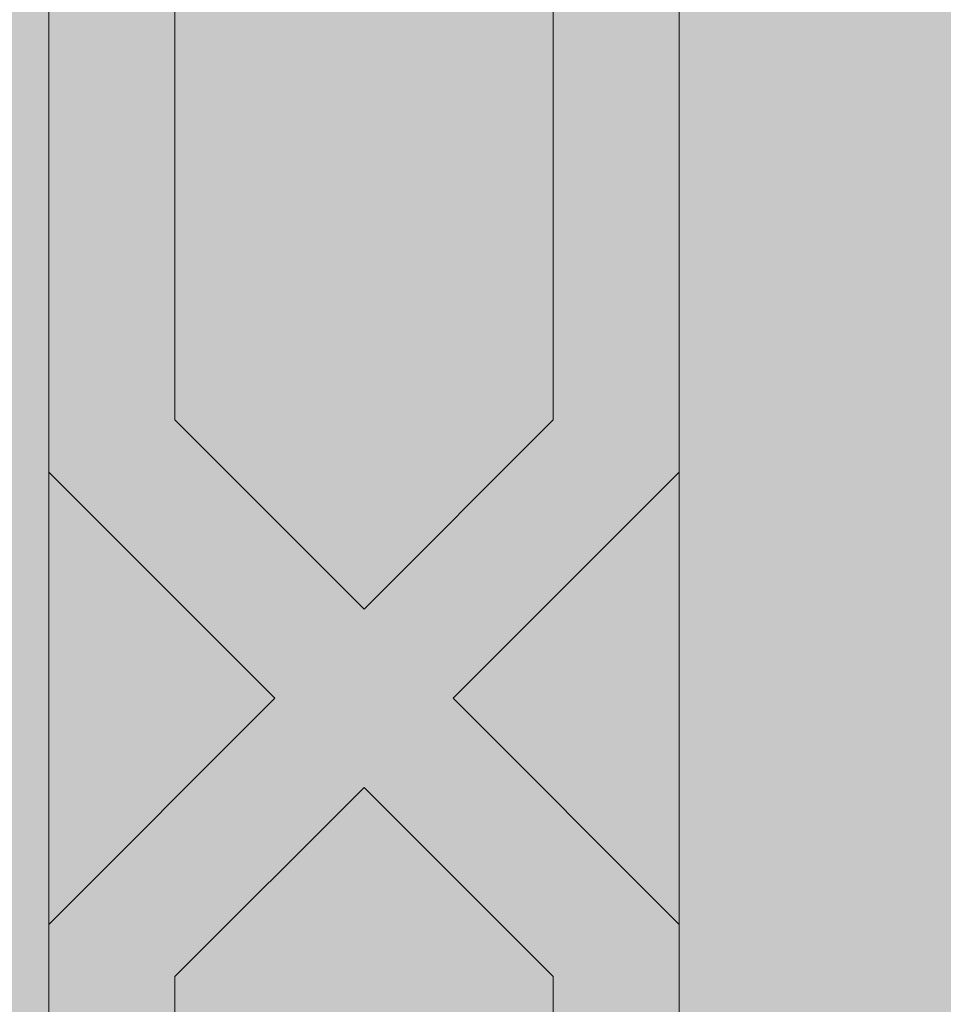
# Model space of a CAD drawing. Units: inches. Extents: x 844 to 2234, y 346 to 1084.
# Tile 17 of 93: x 1116.421 to 1118.29, y 701.25 to 703.242. Entities that reach past the tile are written whole.
import ezdxf

# ---------------------------------------------------------------- set-up
doc = ezdxf.new("R2010")
doc.units = ezdxf.units.IN
doc.header["$MEASUREMENT"] = 0
for name, color, linetype, lineweight in [('A-ANNO-DIMS', 2, 'Continuous', 18), ('furniture', 8, 'Continuous', 18), ('RA-AP-01$0$INT', 35, 'Continuous', 5)]:
    doc.layers.add(name, color=color, linetype=linetype, lineweight=lineweight)
doc.layers.add('RA-AP-01$0$FURN', color=3, linetype='Continuous')
doc.styles.get("Standard").update_dxf_attribs({"font": 'arial.ttf'})
doc.dimstyles.get("Standard").update_dxf_attribs({"dimtxt": 6, "dimasz": 3, "dimexe": 0.18, "dimexo": 0.0625, "dimgap": 0.09, "dimtad": 0, "dimtih": 1, "dimtoh": 1, "dimdec": 1, "dimzin": 0, "dimdsep": 46, "dimlunit": 3, "dimtxsty": 'Standard', "dimblk": 'ARCHTICK', "dimcen": 0.09, "dimadec": 0, "dimazin": 0, "dimtfac": 1, "dimtdec": 1, "dimtofl": 0, "dimtmove": 0, "dimatfit": 3, "dimfxl": 1, "dimtolj": 1, "dimtzin": 0, "dimarcsym": 0})

# ---------------------------------------------------------------- blocks, each defined once
blk = doc.blocks.new('A$C18D01794')
at = {"layer": 'RA-AP-01$0$INT'}
h = blk.add_hatch(color=256, dxfattribs=at)
h.paths.add_polyline_path([(4.355206456958071, -6.156712009588037), (4.355206456958071, -8.056712009588038), (5.455206456958072, -8.056712009588038), (5.455206456958072, -6.156712009588037)])
h.paths.add_polyline_path([(4.405206456958072, -8.006712009588039), (4.405206456958072, -6.206712009588038), (5.405206456958072, -6.206712009588038), (5.405206456958072, -8.006712009588039)], flags=16)
h = blk.add_hatch(color=256, dxfattribs=at)
h.paths.add_polyline_path([(4.505206456958071, -7.585498806127123), (4.46934859260189, -7.549640941759413), (4.505206456958071, -7.513783077414768), (4.505206456958071, -7.381963272220687), (4.469348592616735, -7.346105407867824), (4.505206456958071, -7.310247543514964), (4.505206456958071, -7.178427738324996), (4.469348592586679, -7.142569873965138), (4.505206456952245, -7.106712009588038), (4.476922185709333, -7.106712009588038), (4.455206456960671, -7.128427738343681), (4.433490728198047, -7.106712009588038), (4.405206456946033, -7.106712009588036), (4.441064321339216, -7.142569873969684), (4.40520645695807, -7.178427738362358), (4.405206456958072, -7.310247543472698), (4.441064321364728, -7.346105407867826), (4.40520645695807, -7.381963272262947), (4.40520645695807, -7.513783077378263), (4.441064321354429, -7.549640941786153), (4.405206456958072, -7.585498806170974), (4.405206456958072, -7.717318611286652), (4.441064321333084, -7.753176475673194), (4.405206456958072, -7.789034340036673), (4.405206456958072, -8.006712009588039), (4.644348592588106, -8.006712009588039), (4.680206456964639, -7.970854145211967), (4.716064321341165, -8.006712009588039), (4.869348592586113, -8.006712009588039), (4.905206456964143, -7.970854145210465), (4.941064321342174, -8.006712009588039), (5.094348592587118, -8.006712009588037), (5.130206456963649, -7.970854145211967), (5.166064321340178, -8.006712009588039), (5.405206456958072, -8.006712009588039), (5.405206456958072, -7.789034340024526), (5.369348592595202, -7.753176475673196), (5.40520645695807, -7.717318611298797), (5.40520645695807, -7.585498806158829), (5.369348592573859, -7.549640941786151), (5.40520645695807, -7.51378307739041), (5.40520645695807, -7.381963272250803), (5.36934859256356, -7.346105407867824), (5.405206456958072, -7.310247543484846), (5.405206456958072, -7.178427738350217), (5.369348592589068, -7.142569873969682), (5.405206456982249, -7.106712009588038), (5.376922185730244, -7.106712009588038), (5.355206456967613, -7.128427738343679), (5.333490728218955, -7.10671200958804), (5.305206456976043, -7.106712009588042), (5.341064321341609, -7.142569873965136), (5.305206456958072, -7.178427738337141), (5.305206456958072, -7.310247543502816), (5.34106432131155, -7.346105407867824), (5.305206456958072, -7.381963272232832), (5.30520645695807, -7.513783077402624), (5.341064321326395, -7.549640941759413), (5.305206456958072, -7.585498806139263), (5.305206456958072, -7.717318611299605), (5.341064321347738, -7.753176475677737), (5.305206456958072, -7.78903434007894), (5.30520645695807, -7.906712009588039), (5.166064321336834, -7.906712009588039), (5.130206456963647, -7.942569873961684), (5.094348592590464, -7.906712009588039), (4.941064321338827, -7.906712009588041), (4.905206456964145, -7.942569873963183), (4.869348592589459, -7.906712009588039), (4.716064321337822, -7.906712009588041), (4.680206456964641, -7.942569873961684), (4.644348592591453, -7.906712009588039), (4.505206456958071, -7.906712009588039), (4.505206456958071, -7.789034340066795), (4.469348592580545, -7.753176475677738), (4.505206456958071, -7.717318611311748)])
h.paths.add_polyline_path([(4.485206456974132, -7.709034340046354), (4.45520645695909, -7.739034340051736), (4.425206456974128, -7.709034340057131), (4.425206456993394, -7.593783077384998), (4.45520645699153, -7.563783077396511), (4.485206456993396, -7.593783077408017)], flags=16)
h.paths.add_polyline_path([(4.455206456954537, -7.767318611299197), (4.485206456958242, -7.797318611312542), (4.48520645695951, -7.912569873958716), (4.45520645695415, -7.942569873954422), (4.425206456957888, -7.912569873967813), (4.425206456957888, -7.797318611286197)], flags=16)
h.paths.add_polyline_path([(4.455206456964794, -7.535498806149051), (4.42520645696469, -7.5054988061393), (4.425206456983954, -7.390247543486406), (4.455206456990734, -7.360247543489279), (4.485206456983953, -7.39024754349214), (4.485206456964687, -7.505498806158811)], flags=16)
h.paths.add_polyline_path([(4.499348592588947, -7.926712009585049), (4.636064321340932, -7.926712009585049), (4.666064321342317, -7.956712009586821), (4.636064321343707, -7.986712009585048), (4.499348592575121, -7.986712009585048), (4.469348592591685, -7.956712009591957)], flags=16)
h.paths.add_polyline_path([(4.425206456957888, -7.940854145195974), (4.471064321332215, -7.986712009585049), (4.425206456957888, -7.986712009585049)], flags=16)
h.paths.add_polyline_path([(4.455206456990734, -7.331963272246367), (4.425206456989053, -7.301963272254337), (4.425206456969784, -7.186712009596224), (4.455206456965226, -7.156712009591144), (4.485206456969787, -7.186712009586051), (4.485206456989053, -7.301963272238404)], flags=16)
h.paths.add_polyline_path([(4.72434859258714, -7.926712009586255), (4.861064321340141, -7.926712009586248), (4.891064321340324, -7.956712009586823), (4.861064321340513, -7.986712009586252), (4.724348592586768, -7.986712009586252), (4.694348592586956, -7.956712009586821)], flags=16)
h.paths.add_polyline_path([(4.919348592587961, -7.956712009586821), (4.949348592588145, -7.92671200958625), (5.08606432134115, -7.926712009586253), (5.116064321341327, -7.956712009586823), (5.086064321341519, -7.986712009586252), (4.949348592587774, -7.986712009586252)], flags=16)
h.paths.add_polyline_path([(5.144348592585967, -7.956712009586823), (5.174348592587358, -7.926712009585049), (5.311064321339338, -7.926712009585049), (5.3410643213366, -7.956712009591957), (5.311064321353163, -7.986712009585048), (5.174348592584576, -7.986712009585048)], flags=16)
h.paths.add_polyline_path([(5.32520645693489, -7.593783077408021), (5.355206456936755, -7.563783077396511), (5.385206456934894, -7.593783077384998), (5.38520645695416, -7.709034340057128), (5.355206456969194, -7.739034340051736), (5.325206456954153, -7.709034340046352)], flags=16)
h.paths.add_polyline_path([(5.325206456970042, -7.797318611312542), (5.355206456973747, -7.767318611299197), (5.385206456970398, -7.7973186112862), (5.385206456970398, -7.912569873967816), (5.355206456974136, -7.942569873954422), (5.325206456968778, -7.912569873958716)], flags=16)
h.paths.add_polyline_path([(5.325206456963599, -7.505498806158811), (5.325206456944333, -7.39024754349214), (5.355206456937552, -7.360247543489279), (5.385206456944332, -7.39024754348641), (5.385206456963596, -7.505498806139303), (5.355206456963492, -7.53549880614905)], flags=16)
h.paths.add_polyline_path([(5.32520645693923, -7.301963272238403), (5.3252064569585, -7.186712009586051), (5.355206456963062, -7.156712009591142), (5.3852064569585, -7.186712009596224), (5.385206456939234, -7.301963272254338), (5.355206456937552, -7.331963272246369)], flags=16)
h.paths.add_polyline_path([(5.339348592596071, -7.986712009585048), (5.385206456970398, -7.940854145195972), (5.385206456970396, -7.986712009585048)], flags=16)
h = blk.add_hatch(color=256, dxfattribs=at)
h.paths.add_polyline_path([(4.469348592586677, -7.142569873965136), (4.505206456958073, -7.178427738324996), (4.505206456958071, -7.106712009582215)])
h.paths.add_polyline_path([(4.455206456960671, -7.128427738343681), (4.476922185709333, -7.106712009588038), (4.433490728198045, -7.106712009588038)])
h.paths.add_polyline_path([(4.405206456958073, -7.178427738362358), (4.441064321339218, -7.142569873969684), (4.40520645695807, -7.106712009600073)])
h.paths.add_polyline_path([(4.425206456989053, -7.301963272254335), (4.455206456990736, -7.331963272246371), (4.485206456989055, -7.301963272238399), (4.48520645696979, -7.186712009586054), (4.455206456965227, -7.15671200959114), (4.425206456969784, -7.186712009596224)])
h.paths.add_polyline_path([(4.505206456958073, -7.381963272220689), (4.505206456958071, -7.310247543514961), (4.469348592616738, -7.346105407867826)])
h.paths.add_polyline_path([(4.425206456964688, -7.5054988061393), (4.455206456964794, -7.535498806149051), (4.485206456964689, -7.505498806158811), (4.485206456983951, -7.390247543492138), (4.455206456990736, -7.360247543489277), (4.425206456983956, -7.39024754348641)])
h.paths.add_polyline_path([(4.425206456974126, -7.709034340057128), (4.455206456959092, -7.739034340051736), (4.485206456974132, -7.709034340046356), (4.485206456993396, -7.593783077408017), (4.45520645699153, -7.563783077396511), (4.425206456993394, -7.593783077384999)])
h.paths.add_polyline_path([(4.46934859260189, -7.549640941759415), (4.505206456958071, -7.585498806127123), (4.505206456958073, -7.513783077414766)])
h.paths.add_polyline_path([(4.405206456958073, -7.585498806170972), (4.441064321354427, -7.549640941786151), (4.405206456958072, -7.513783077378263)])
h.paths.add_polyline_path([(4.405206456958072, -7.789034340036673), (4.441064321333084, -7.753176475673194), (4.405206456958072, -7.71731861128665)])
h.paths.add_polyline_path([(4.469348592580547, -7.75317647567774), (4.505206456958071, -7.789034340066795), (4.505206456958071, -7.717318611311744)])
h.paths.add_polyline_path([(4.425206456957888, -7.912569873967814), (4.45520645695415, -7.942569873954422), (4.485206456959507, -7.912569873958718), (4.48520645695824, -7.797318611312542), (4.455206456954537, -7.767318611299197), (4.425206456957888, -7.797318611286202)])
h.paths.add_polyline_path([(4.425206456957888, -7.986712009585049), (4.471064321332215, -7.986712009585049), (4.425206456957888, -7.940854145195972)])
h.paths.add_polyline_path([(4.499348592575121, -7.986712009585048), (4.636064321343707, -7.986712009585049), (4.666064321342317, -7.956712009586823), (4.636064321340932, -7.926712009585049), (4.499348592588945, -7.926712009585049), (4.469348592591685, -7.95671200959196)])
h.paths.add_polyline_path([(4.680206456964641, -7.942569873961684), (4.716064321337824, -7.906712009588039), (4.644348592591454, -7.906712009588039)])
h.paths.add_polyline_path([(4.644348592588108, -8.006712009588039), (4.716064321341167, -8.006712009588039), (4.680206456964637, -7.970854145211964)])
h.paths.add_polyline_path([(4.724348592586768, -7.98671200958625), (4.861064321340514, -7.986712009586252), (4.891064321340324, -7.956712009586819), (4.861064321340141, -7.92671200958625), (4.724348592587134, -7.926712009586255), (4.694348592586957, -7.956712009586821)])
h.paths.add_polyline_path([(4.905206456964143, -7.942569873963183), (4.941064321338827, -7.906712009588039), (4.869348592589457, -7.906712009588037)])
h.paths.add_polyline_path([(4.869348592586113, -8.006712009588039), (4.941064321342172, -8.006712009588037), (4.905206456964145, -7.970854145210463)])
h.paths.add_polyline_path([(4.949348592587774, -7.986712009586252), (5.086064321341521, -7.986712009586252), (5.116064321341329, -7.956712009586823), (5.08606432134115, -7.926712009586253), (4.949348592588145, -7.92671200958625), (4.919348592587961, -7.956712009586819)])
h.paths.add_polyline_path([(5.130206456963645, -7.942569873961684), (5.166064321336834, -7.906712009588039), (5.094348592590464, -7.906712009588039)])
h.paths.add_polyline_path([(5.094348592587119, -8.006712009588039), (5.166064321340178, -8.006712009588039), (5.130206456963651, -7.970854145211967)])
h.paths.add_polyline_path([(5.174348592584578, -7.986712009585048), (5.311064321353163, -7.986712009585048), (5.341064321336602, -7.956712009591958), (5.31106432133934, -7.926712009585049), (5.174348592587352, -7.926712009585049), (5.144348592585969, -7.956712009586823)])
h.paths.add_polyline_path([(5.325206456968778, -7.912569873958718), (5.355206456974136, -7.942569873954422), (5.385206456970396, -7.912569873967814), (5.385206456970396, -7.797318611286199), (5.355206456973747, -7.767318611299197), (5.325206456970044, -7.797318611312544)])
h.paths.add_polyline_path([(5.339348592596073, -7.986712009585048), (5.385206456970396, -7.986712009585049), (5.385206456970398, -7.94085414519597)])
h.paths.add_polyline_path([(5.325206456954155, -7.709034340046354), (5.355206456969194, -7.739034340051734), (5.38520645695416, -7.709034340057128), (5.385206456934896, -7.593783077384999), (5.355206456936758, -7.563783077396513), (5.325206456934888, -7.593783077408019)])
h.paths.add_polyline_path([(5.305206456958072, -7.789034340078938), (5.341064321347739, -7.753176475677738), (5.305206456958072, -7.717318611299605)])
h.paths.add_polyline_path([(5.369348592595204, -7.753176475673194), (5.40520645695807, -7.789034340024526), (5.405206456958072, -7.717318611298798)])
h.paths.add_polyline_path([(5.405206456958072, -7.585498806158831), (5.405206456958072, -7.513783077390407), (5.369348592573857, -7.549640941786151)])
h.paths.add_polyline_path([(5.305206456958072, -7.585498806139266), (5.341064321326393, -7.549640941759413), (5.305206456958072, -7.513783077402626)])
h.paths.add_polyline_path([(5.325206456963599, -7.50549880615881), (5.355206456963494, -7.535498806149055), (5.385206456963598, -7.505498806139302), (5.385206456944334, -7.390247543486411), (5.355206456937552, -7.360247543489279), (5.325206456944333, -7.39024754349214)])
h.paths.add_polyline_path([(5.305206456958072, -7.38196327223283), (5.341064321311551, -7.346105407867824), (5.305206456958072, -7.31024754350282)])
h.paths.add_polyline_path([(5.325206456939231, -7.301963272238404), (5.355206456937552, -7.331963272246369), (5.385206456939235, -7.301963272254335), (5.385206456958502, -7.186712009596224), (5.355206456963061, -7.156712009591142), (5.3252064569585, -7.186712009586051)])
h.paths.add_polyline_path([(5.404581768715993, -7.381338584008926, -0.001217816984214), (5.405206456958072, -7.381112009582329), (5.405206456958072, -7.310247543484846), (5.369348592563558, -7.346105407867826)])
h.paths.add_polyline_path([(5.36934859258907, -7.142569873969684), (5.40520645695807, -7.178427738350215), (5.405206456958072, -7.106712009612218)])
h.paths.add_polyline_path([(5.355206456967613, -7.128427738343683), (5.376922185730239, -7.106712009588038), (5.333490728218953, -7.10671200958804)])
h.paths.add_polyline_path([(5.30520645695807, -7.178427738337139), (5.341064321341609, -7.142569873965134), (5.305206456958074, -7.10671200957007)])
blk.add_hatch(color=256, dxfattribs=at).paths.add_polyline_path([(4.505206456958071, -7.906712009588039), (5.305206456958072, -7.906712009588039), (5.305206456958072, -7.106712009588038), (5.255206456951893, -7.106712009588036), (5.25520645694868, -7.856712009570104), (4.555206456959269, -7.856712009588616), (4.555206456956052, -7.106712009588038), (4.505206456958073, -7.106712009588038)])
for p, q in [((4.425206456983954, -7.39024754348641), (4.425206456964688, -7.5054988061393)), ((4.485206456983953, -7.39024754349214), (4.485206456964687, -7.505498806158811)), ((4.425206456964688, -7.5054988061393), (4.455206456964796, -7.535498806149051)), ((4.485206456964687, -7.505498806158811), (4.455206456964796, -7.535498806149051)), ((4.405206456968717, -7.513783077388909), (4.441064321338788, -7.54964094177051)), ((4.505206456968717, -7.513783077404122), (4.469348592586251, -7.549640941775054)), ((4.405206456988469, -7.585498806140577), (4.441064321370071, -7.549640941770508)), ((4.505206456988468, -7.58549880615752), (4.469348592617532, -7.549640941775056)), ((4.425206456993394, -7.593783077384996), (4.45520645699153, -7.563783077396511)), ((4.485206456993396, -7.593783077408017), (4.45520645699153, -7.563783077396511)), ((4.425206456993394, -7.593783077384996), (4.425206456974128, -7.709034340057129)), ((4.485206456993396, -7.593783077408017), (4.485206456974132, -7.709034340046354))]:
    blk.add_line(p, q, dxfattribs=at)
for points in [[(5.405206456958072, -8.006712009588039), (4.405206456958072, -8.006712009588039), (4.405206456958072, -7.106712009588038)], [(5.305206456958072, -7.106712009588038), (5.305206456958072, -7.906712009588039), (4.505206456958071, -7.906712009588039), (4.505206456958071, -7.106712009588038)]]:
    blk.add_lwpolyline(points, dxfattribs=at)
blk = doc.blocks.new('A$C5D2F253E')
at = {"layer": 'RA-AP-01$0$FURN', "xscale": -0.7999999999883585, "yscale": 0.7999999999883585, "zscale": 0.8, "rotation": 90}
blk.add_blockref('A$C18D01794', (-5.687757199772477, 4.75791982714071), dxfattribs=at)
blk = doc.blocks.new('_ArchTick')
at = {"color": 0, "linetype": 'ByBlock', "const_width": 0.15}
blk.add_lwpolyline([(-0.5, -0.5), (0.5, 0.5)], dxfattribs=at)
blk = doc.blocks.new('*D144')
at = {"layer": 'A-ANNO-DIMS', "color": 0, "lineweight": -2, "transparency": 16777216}
for p, q in [((1096.615948, 439.3732739999999), (1096.615948, 1074.743301)), ((1143.115948, 492.373274), (1143.115948, 1074.743301)), ((1096.615948, 1074.563301), (1102.481950728513, 1074.563301)), ((1143.115948, 1074.563301), (1137.249945271487, 1074.563301))]:
    blk.add_line(p, q, dxfattribs=at)
at = {"layer": 'Defpoints', "color": 0, "transparency": 16777216}
for p in [(1143.115948, 1074.563301), (1143.115948, 492.3107739999999), (1096.615948, 439.3107739999999)]:
    blk.add_point(p, dxfattribs=at)
at = {"layer": 'A-ANNO-DIMS', "color": 0, "lineweight": -2, "transparency": 16777216, "xscale": 3, "yscale": 3, "zscale": 3, "rotation": 180}
blk.add_blockref('_ArchTick', (1096.615948, 1074.563301), dxfattribs=at)
at = {"layer": 'A-ANNO-DIMS', "color": 0, "lineweight": -2, "transparency": 16777216, "xscale": 3, "yscale": 3, "zscale": 3}
blk.add_blockref('_ArchTick', (1143.115948, 1074.563301), dxfattribs=at)
at = {"layer": 'A-ANNO-DIMS', "color": 0, "transparency": 16777216, "insert": (1119.865948, 1074.563301), "char_height": 6, "attachment_point": 5}
blk.add_mtext('\\A1;3\'-10 1/2"', dxfattribs=at)

msp = doc.modelspace()

# ---------------------------------------------------------------- block references
at = {"layer": 'furniture', "xscale": 15.94108302203742, "yscale": 15.94108302203742, "zscale": 15.94108302203742, "rotation": 90}
msp.add_blockref('A$C5D2F253E', (1136.147844094663, 696.2584716700112), dxfattribs=at)

# ---------------------------------------------------------------- dimensions: what is measured, and where the dimension line sits
at = {"layer": 'A-ANNO-DIMS'}
dim = msp.add_linear_dim(base=(1143.115948, 1074.563301), p1=(1096.615948, 439.3107739999999), p2=(1143.115948, 492.3107739999999), dimstyle='Standard', override={"dimdec": 1, "dimlfac": 1, "dimrnd": 0, "dimzin": 1, "dimdsep": 46, "dimlunit": 4, "dimfrac": 2}, dxfattribs=at)
dim.commit()
dim.dimension.update_dxf_attribs({"geometry": '*D144', "text_midpoint": (1119.865948, 1074.563301)})

doc.saveas('drawing.dxf')
